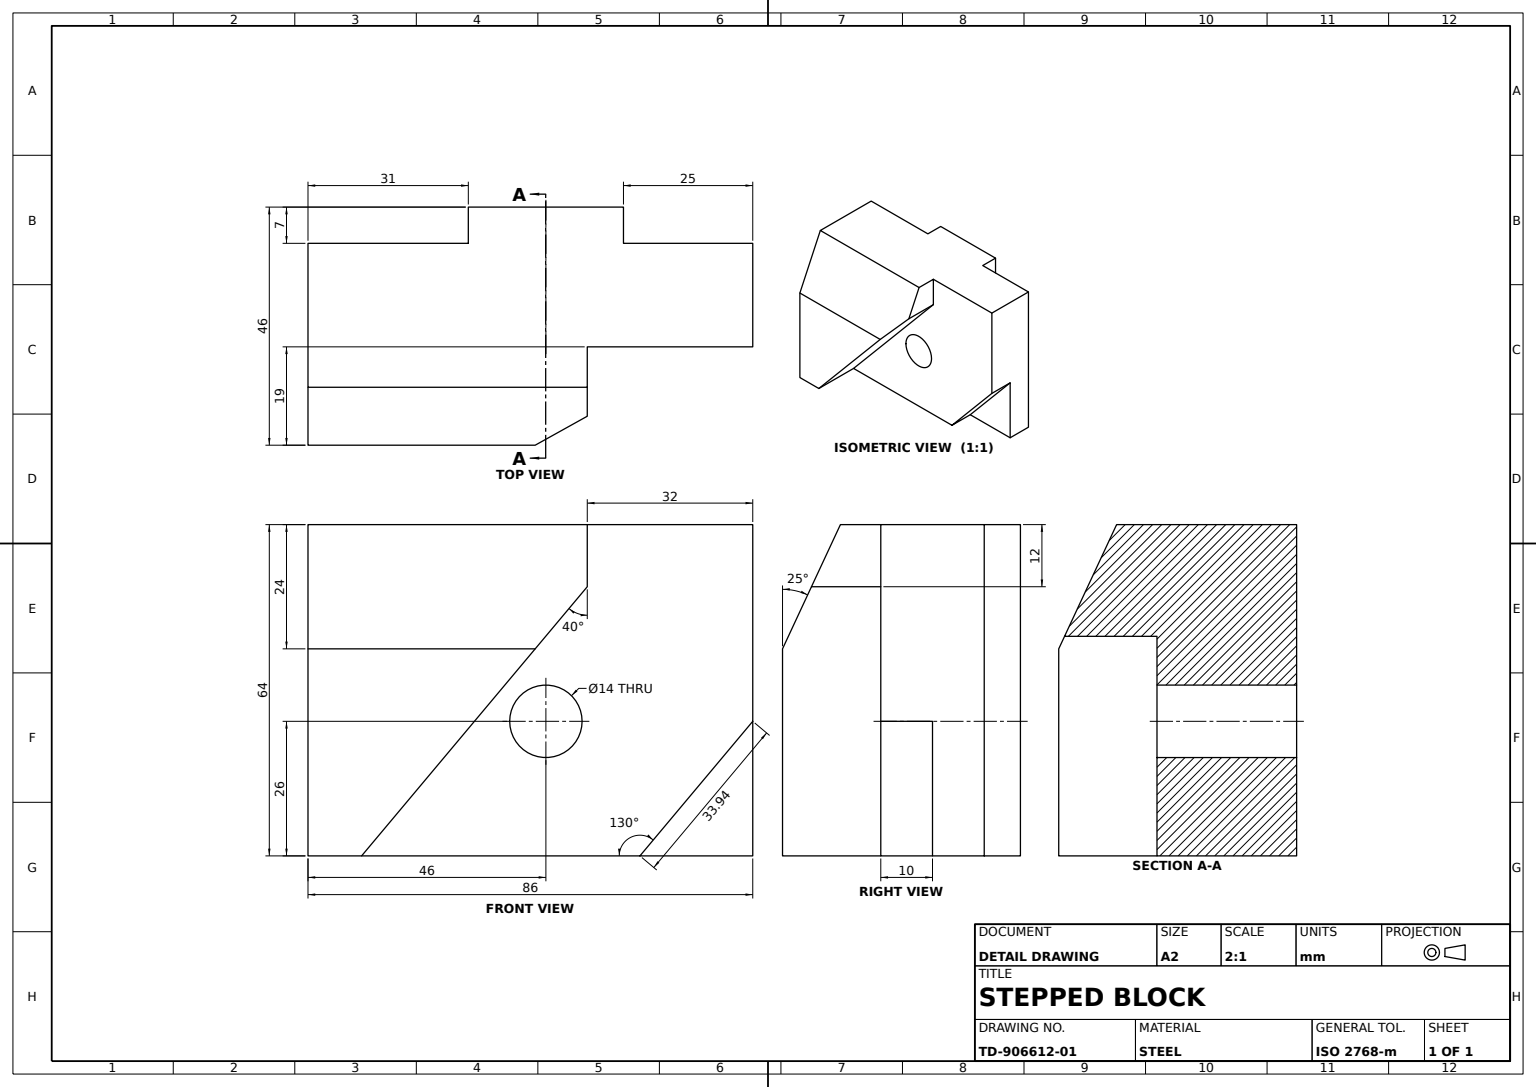
from build123d import *

# Parameters (mm, degrees)
BASE_PLATE_SKETCH_W        = 86
BASE_PLATE_SKETCH_H        = 64
BASE_PLATE_86X64X10_DEPTH  = 10
UPPER_LAYER_SKETCH_W       = 86
UPPER_LAYER_SKETCH_H       = 64
UPPER_LAYER_BOSS_10_DEPTH  = 10
ANGLED_STEP_BOSS_19_DEPTH  = 19
ANGLED_CUT_25DEG_DEPTH     = 65
THROUGH_HOLE_SKETCH_R      = 7
THROUGH_HOLE_14_DEPTH      = 65
TRIANGULAR_NOTCH_CUT_DEPTH = 10
SIDE_BOSS_SKETCH_W         = 30
SIDE_BOSS_SKETCH_H         = 7
SIDE_BOSS_64_DEPTH         = 64
SIDE_BOSS_HOLE_SKETCH_R    = 7
SIDE_BOSS_HOLE_14_DEPTH    = 64


with BuildPart() as part:
    # Base Plate Sketch → Base Plate 86x64x10 (new body)
    with BuildSketch(Plane.XY):
        with Locations((43, 32)):
            Rectangle(BASE_PLATE_SKETCH_W, BASE_PLATE_SKETCH_H)
    extrude(amount=BASE_PLATE_86X64X10_DEPTH)

    # Upper Layer Sketch → Upper Layer Boss 10 (add)
    with BuildSketch(Plane.XY.offset(10)):
        with Locations((43, 32)):
            Rectangle(UPPER_LAYER_SKETCH_W, UPPER_LAYER_SKETCH_H)
    extrude(amount=UPPER_LAYER_BOSS_10_DEPTH)

    # Angled Step Sketch → Angled Step Boss 19 (add)
    with BuildSketch(Plane.XY.offset(20)):
        Polygon((54, 52), (54, 64), (0, 64), (0, 0), (10.366819179, 0), align=None)
    extrude(amount=ANGLED_STEP_BOSS_19_DEPTH)

    # Angled Cut Sketch → Angled Cut 25deg (cut)
    with BuildSketch(Plane.ZY):
        Polygon((39, 64), (39, 40), (27.808616204, 64), align=None)
    extrude(amount=-ANGLED_CUT_25DEG_DEPTH, mode=Mode.SUBTRACT)

    # Through Hole Sketch → Through Hole Ø14 (cut)
    with BuildSketch(Plane.XY.offset(20)):
        with Locations((46, 26)):
            Circle(THROUGH_HOLE_SKETCH_R)
    extrude(amount=-THROUGH_HOLE_14_DEPTH, mode=Mode.SUBTRACT)

    # Triangular Notch Sketch → Triangular Notch Cut (cut)
    with BuildSketch(Plane.XY.offset(20)):
        Polygon((86, 0), (86, 26), (64.183409589, 0), align=None)
    extrude(amount=-TRIANGULAR_NOTCH_CUT_DEPTH, mode=Mode.SUBTRACT)

    # Side Boss Sketch → Side Boss 64 (add)
    with BuildSketch(Plane.XZ):
        with Locations((46, -3.5)):
            Rectangle(SIDE_BOSS_SKETCH_W, SIDE_BOSS_SKETCH_H)
    extrude(amount=-SIDE_BOSS_64_DEPTH)

    # Side Boss Hole Sketch → Side Boss Hole Ø14 (cut)
    with BuildSketch(Plane.XY):
        with Locations((46, 26)):
            Circle(SIDE_BOSS_HOLE_SKETCH_R)
    extrude(amount=-SIDE_BOSS_HOLE_14_DEPTH, mode=Mode.SUBTRACT)


solid = part.part
